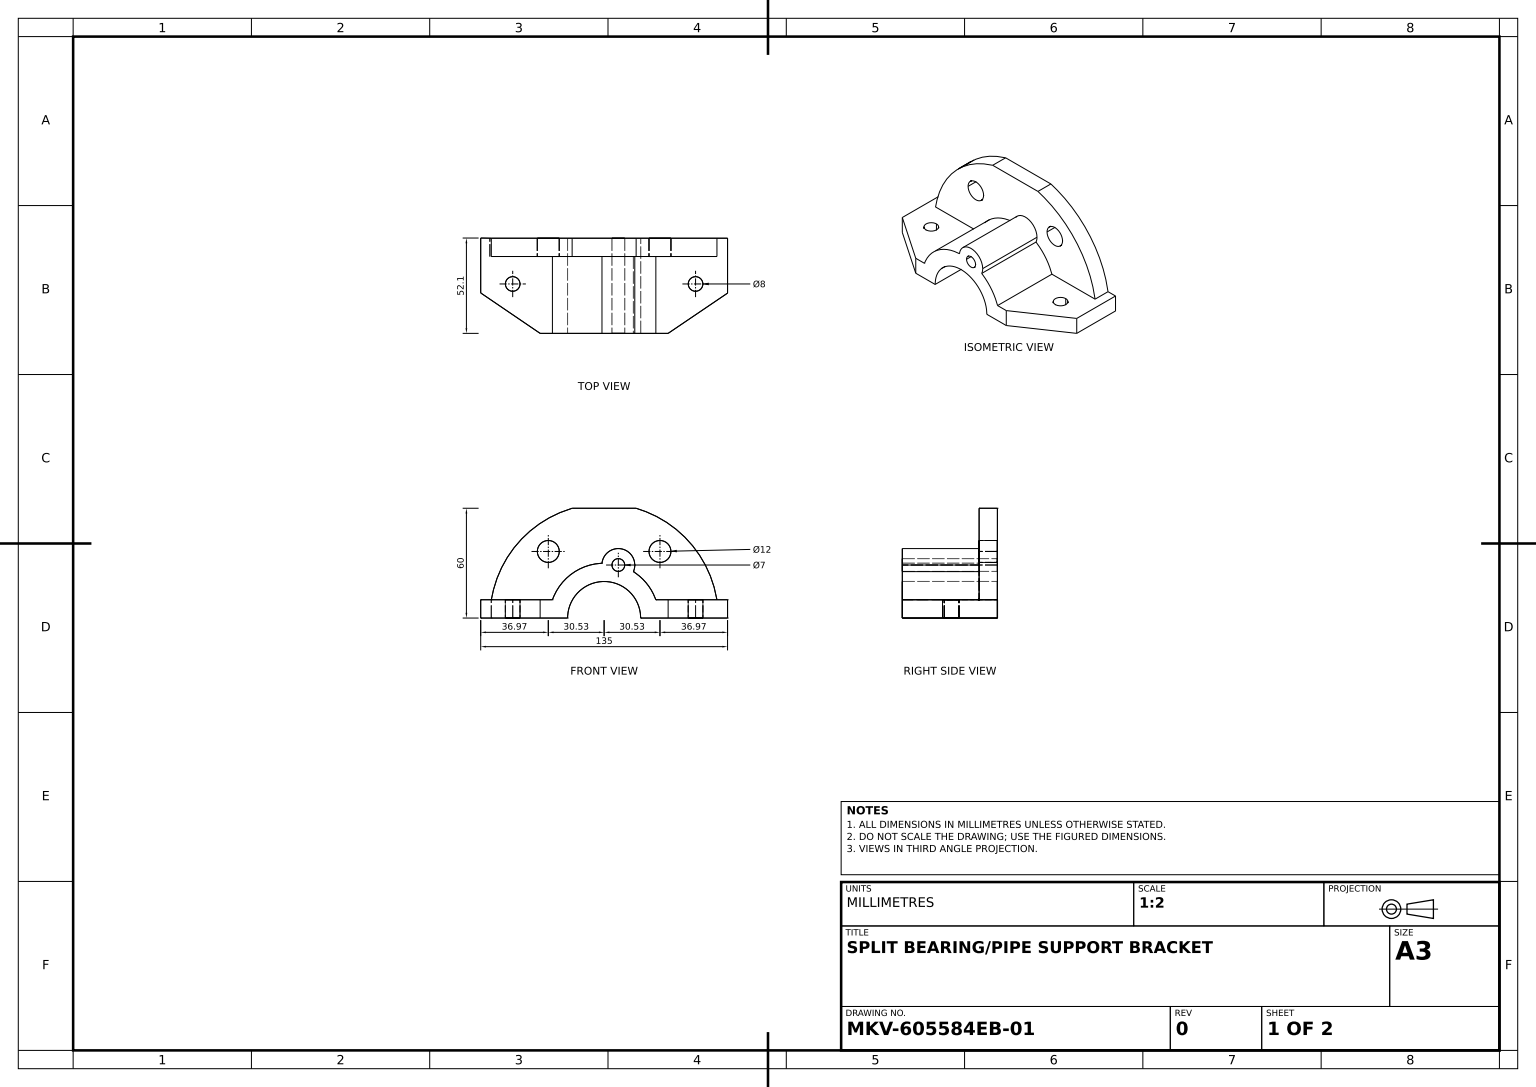
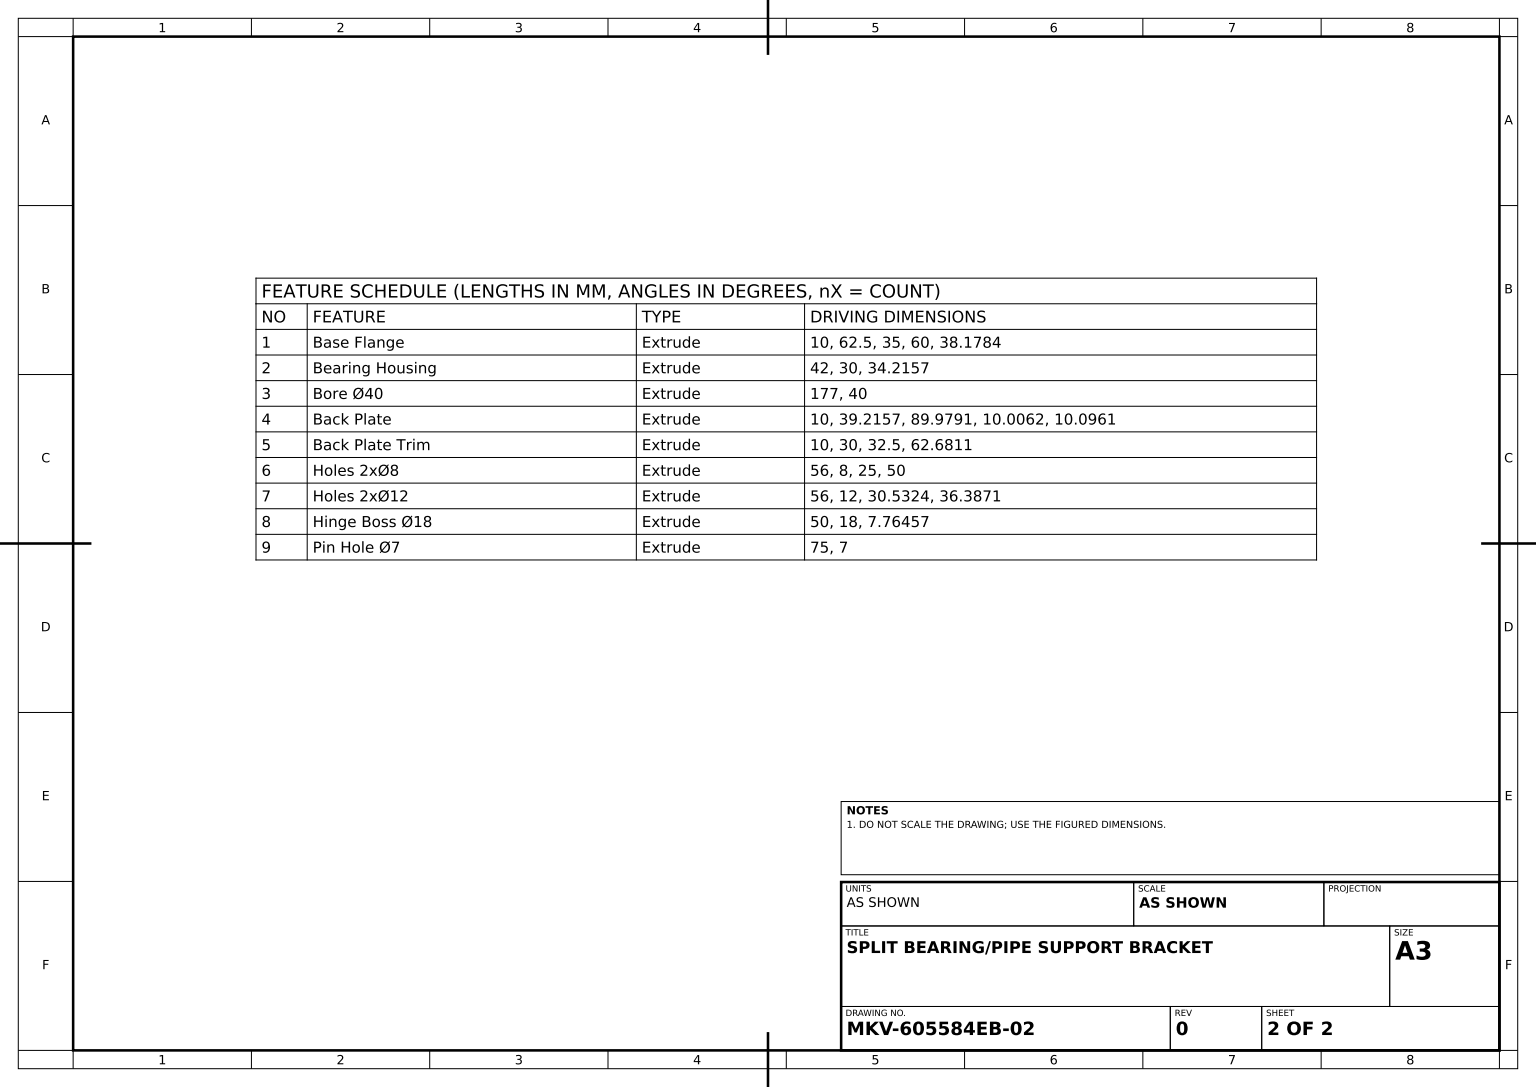
SolidWorks part; units mm, degrees
material "Plain Carbon Steel"
ref_plane "Front Plane" through (0, 0, 0) normal (0, 0, 1) x (1, 0, 0)
ref_plane "Top Plane" through (0, 0, 0) normal (0, 1, 0) x (1, 0, 0)
ref_plane "Right Plane" through (0, 0, 0) normal (1, 0, 0) x (0, 0, -1)
sketch "Base Flange Sketch" plane through (0, 0, 0) normal (0, 0, 1) x (1, 0, 0)
  line L0 (0, 0) -> (38.1784, 0)
  line L2 (0, 60) -> (17.5, 60)
  line L3 (0, 60) -> (-17.5, 60)
  line L4 (-62.5, 0) -> (62.5, 0)
  arc A0 (-17.5, 60) -> (-62.5, 0) centre (0, 0) ccw
  arc A1 (62.5, 0) -> (17.5, 60) centre (0, 0) ccw
  dimension "D1" = 62.5
  dimension "D2" = 35
  dimension "D3" = 60
  dimension "D4" = 38.1784
extrude "Base Flange" add sketch "Base Flange Sketch" along normal blind 10 contours L4 A1 L2 L3 A0 L0
sketch "Bearing Housing Sketch" plane through (0, 0, 10) normal (0, 0, 1) x (1, 0, 0)
  line L0 (62.5, 0) -> (62.5, 10)
  line L1 (62.5, 10) -> (28.2843, 10)
  line L2 (-62.5, 10) -> (-62.5, 0)
  line L3 (30, 0) -> (62.5, 0)
  line L4 (-30, 0) -> (-62.5, 0)
  line L5 (-28.2843, 10) -> (-62.5, 10)
  arc A0 (30, 0) -> (-30, 0) centre (0, 0) ccw
  line M3 (-62.5, 0) -> (62.5, 0)
  arc M4 (62.5, 0) -> (17.5, 60) centre (0, 0) ccw
  arc M6 (-17.5, 60) -> (-62.5, 0) centre (0, 0) ccw
  dimension "D1" = 30
  dimension "D2" = 34.2157
extrude "Bearing Housing" add sketch "Bearing Housing Sketch" along normal blind 42 contours A0 L1 M3 M4 | A0 M3 | A0 L5 M6 M3
sketch "Bore Ø40 Sketch" plane through (0, 0, 52) normal (0, 0, 1) x (1, 0, 0)
  circle A0 centre (0, 0) radius 20
  dimension "D1" = 40
extrude "Bore Ø40" cut sketch "Bore Ø40 Sketch" against normal blind 177
sketch "Back Plate Sketch" plane through (0, 10, 0) normal (0, 1, 0) x (1, 0, 0)
  line L0 (61.6948, -52) -> (67.5, -52)
  line L1 (28.2843, -52) -> (28.2843, -10) construction
  line L2 (67.5, -52) -> (67.5, 0)
  line L3 (67.5, 0) -> (62.5, 0)
  line L5 (-67.5, -52) -> (-61.6948, -52)
  line L6 (-67.5, 0.0961) -> (-61.6948, 0.0062)
  line L7 (-61.6948, 0.0062) -> (-61.6948, -52)
  line L8 (-67.5, -52) -> (-67.5, 0.0961)
  line L9 (61.6948, -52) -> (61.6948, 0)
  line L10 (62.5, 0) -> (17.5, 0) construction
  line L11 (61.6948, 0) -> (62.5, 0)
  line L12 (61.6948, -10) -> (28.2843, -10) construction
  dimension "D1" = 39.2157
  dimension "D2" = 89.9791
  dimension "D3" = 10.0062
  dimension "D4" = 10.0961
extrude "Back Plate" add sketch "Back Plate Sketch" against normal blind 10
sketch "Back Plate Trim Sketch" plane through (0, 10, 0) normal (0, 1, 0) x (1, 0, 0)
  line L0 (67.5, 0) -> (67.5, -30)
  line L1 (67.5, -52) -> (67.5, 0) construction
  line L2 (0, -52) -> (35, -52)
  line L3 (-28.2843, -52) -> (28.2843, -52) construction
  line L4 (67.5, -52) -> (28.2843, -52) construction
  line L5 (35, -52) -> (67.5, -30)
  line L6 (-67.5, 0.0961) -> (-67.5, -29.9039)
  line L7 (-67.5, 0.0961) -> (-67.5, -52) construction
  line L8 (0, -52) -> (-35, -52)
  line L9 (-28.2843, -52) -> (-67.5, -52) construction
  line L10 (-67.5, -29.9039) -> (-35, -52)
  line L11 (67.5, -30) -> (67.5, -52)
  line L12 (67.5, -52) -> (35, -52)
  line L13 (-35, -52) -> (-67.5, -52)
  line L14 (-67.5, -52) -> (-67.5, -29.9039)
  line M6 (28.2843, -52) -> (67.5, -52)
  line M7 (67.5, -52) -> (67.5, 0)
  dimension "D1" = 30
  dimension "D2" = 32.5
  dimension "D3" = 32.5
  dimension "D4" = 62.6811
extrude "Back Plate Trim" cut sketch "Back Plate Trim Sketch" against normal blind 10 contours L5 M6 M7 | L14 L13 L10
sketch "Holes 2xØ8 Sketch" plane through (0, 10, 0) normal (0, 1, 0) x (1, 0, 0)
  circle A0 centre (50, -25) radius 4
  circle A1 centre (-50, -25) radius 4
  dimension "D1" = 8
  dimension "D2" = 8
  dimension "D3" = 25
  dimension "D4" = 50
  dimension "D5" = 50
  dimension "D6" = 25
extrude "Holes 2xØ8" cut sketch "Holes 2xØ8 Sketch" against normal blind 56
sketch "Holes 2xØ12 Sketch" plane through (0, 0, 10) normal (0, 0, 1) x (1, 0, 0)
  circle A1 centre (30.5324, 36.3871) radius 6
  circle A2 centre (-30.5324, 36.3871) radius 6
  dimension "D1" = 12
  dimension "D4" = 12
  dimension "D2" = 30.5324
  dimension "D3" = 36.3871
  dimension "D5" = 36.3871
  dimension "D6" = 30.5324
extrude "Holes 2xØ12" cut sketch "Holes 2xØ12 Sketch" against normal blind 56
sketch "Hinge Boss Ø18 Sketch" plane through (0, 0, 52) normal (0, 0, 1) x (1, 0, 0)
  circle A0 centre (7.7646, 28.9778) radius 9
  arc A1 (28.2843, 10) -> (-28.2843, 10) centre (0, 0) ccw construction
  dimension "D1" = 18
  dimension "D2" = 7.7646
extrude "Hinge Boss Ø18" add sketch "Hinge Boss Ø18 Sketch" against normal blind 50
sketch "Pin Hole Ø7 Sketch" plane through (0, 0, 52) normal (0, 0, 1) x (1, 0, 0)
  circle A0 centre (7.7646, 28.9778) radius 3.5
  dimension "D1" = 7
extrude "Pin Hole Ø7" cut sketch "Pin Hole Ø7 Sketch" against normal blind 75
